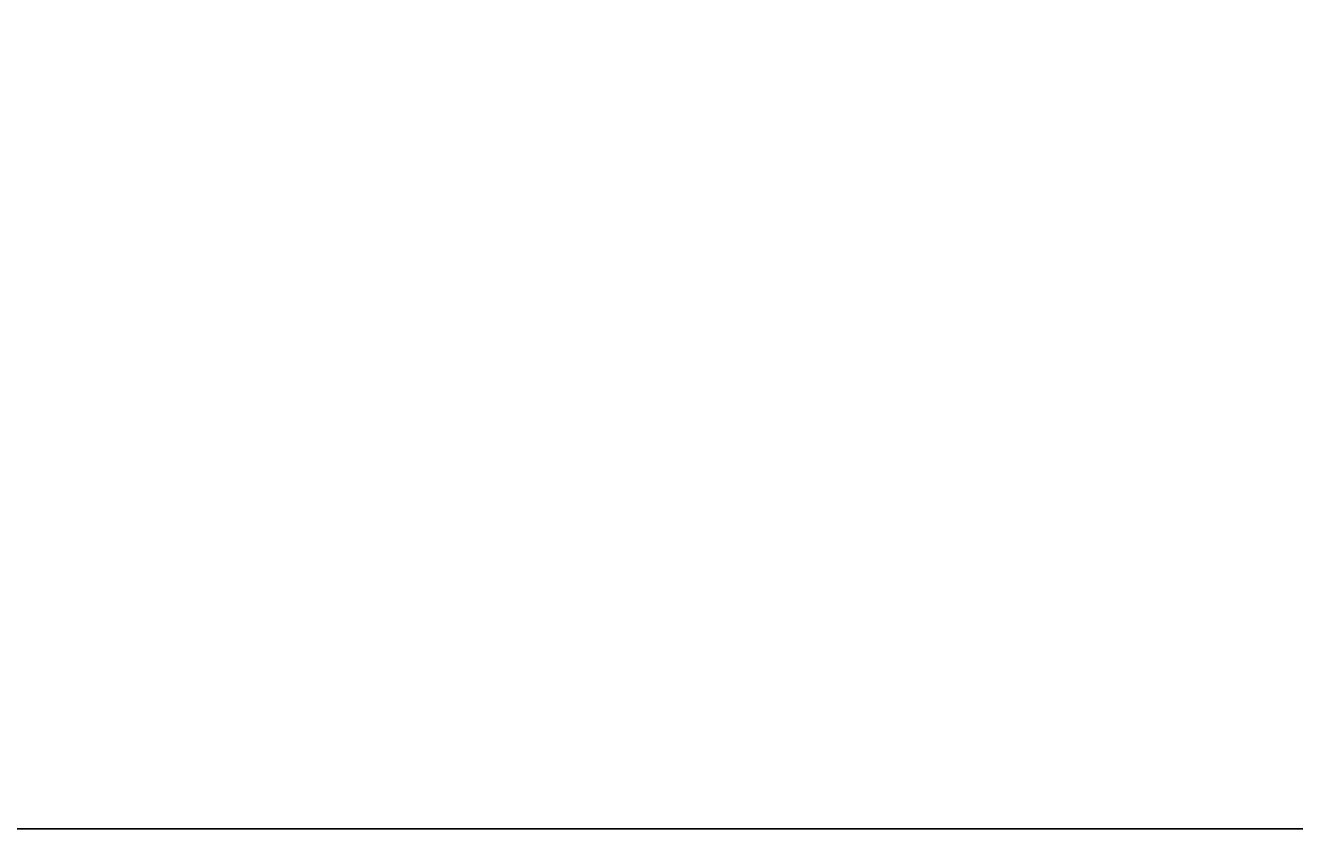
# Model space of a CAD drawing. Units: inches. Extents: x 35362 to 73946, y 43607 to 67532.
# Tile 108 of 134: x 50761 to 50905, y 48969 to 49061. Entities that reach past the tile are written whole.
import ezdxf

# ---------------------------------------------------------------- set-up
doc = ezdxf.new("R2010")
doc.units = ezdxf.units.IN
doc.header["$MEASUREMENT"] = 0
doc.layers.add('A-ANNO-DIMS', color=2, linetype='Continuous', lineweight=18)
doc.styles.get("Standard").update_dxf_attribs({"font": 'arial.ttf'})
doc.dimstyles.get("Standard").update_dxf_attribs({"dimtxt": 0.18, "dimasz": 0.18, "dimexe": 0.18, "dimexo": 0.0625, "dimgap": 0.09, "dimtad": 0, "dimtih": 1, "dimtoh": 1, "dimdec": 4, "dimzin": 0, "dimdsep": 46, "dimtxsty": 'Standard', "dimcen": 0.09, "dimadec": 0, "dimazin": 0, "dimtfac": 1, "dimtdec": 4, "dimtofl": 0, "dimtmove": 0, "dimatfit": 3, "dimfxl": 1, "dimtolj": 1, "dimtzin": 0, "dimarcsym": 0})

# ---------------------------------------------------------------- blocks, each defined once
blk = doc.blocks.new('*D11')
at = {"layer": 'A-ANNO-DIMS', "color": 0, "lineweight": -2, "transparency": 16777216}
for p, q in [((47978.66, 56028.77), (47978.66, 43606.68)), ((53109.76, 56028.77), (53109.76, 43606.68)), ((47978.84, 43606.86), (50543.87, 43606.86)), ((53109.58, 43606.86), (50544.55, 43606.86))]:
    blk.add_line(p, q, dxfattribs=at)
at = {"layer": 'A-ANNO-DIMS', "color": 0, "transparency": 16777216}
for points in [[(47978.84, 43606.89), (47978.84, 43606.83), (47978.66, 43606.86)], [(53109.58, 43606.89), (53109.58, 43606.83), (53109.76, 43606.86)]]:
    blk.add_solid(points, dxfattribs=at)
at = {"layer": 'Defpoints', "color": 0, "transparency": 16777216}
for p in [(47978.66, 56028.84), (53109.76, 56028.84), (53109.76, 43606.86)]:
    blk.add_point(p, dxfattribs=at)
at = {"layer": 'A-ANNO-DIMS', "color": 0, "transparency": 16777216, "insert": (50544.21, 43606.86), "char_height": 0.18, "attachment_point": 5}
blk.add_mtext('\\A1;5131', dxfattribs=at)
blk = doc.blocks.new('*D13')
at = {"layer": 'A-ANNO-DIMS', "color": 0, "lineweight": -2, "transparency": 16777216}
for p, q in [((48373.49, 51694.02), (48373.49, 43606.68)), ((51029.04, 51694.02), (51029.04, 43606.68)), ((48373.67, 43606.86), (49700.8, 43606.86)), ((51028.86, 43606.86), (49701.73, 43606.86))]:
    blk.add_line(p, q, dxfattribs=at)
at = {"layer": 'A-ANNO-DIMS', "color": 0, "transparency": 16777216}
for points in [[(48373.67, 43606.89), (48373.67, 43606.83), (48373.49, 43606.86)], [(51028.86, 43606.89), (51028.86, 43606.83), (51029.04, 43606.86)]]:
    blk.add_solid(points, dxfattribs=at)
at = {"layer": 'Defpoints', "color": 0, "transparency": 16777216}
for p in [(48373.49, 51694.09), (51029.04, 51694.09), (51029.04, 43606.86)]:
    blk.add_point(p, dxfattribs=at)
at = {"layer": 'A-ANNO-DIMS', "color": 0, "transparency": 16777216, "insert": (49701.27, 43606.86), "char_height": 0.18, "attachment_point": 5}
blk.add_mtext('\\A1;2655.6', dxfattribs=at)
blk = doc.blocks.new('*D17')
at = {"layer": 'A-ANNO-DIMS', "color": 0, "lineweight": -2, "transparency": 16777216}
for p, q in [((49923.31, 61293.22), (49923.31, 43606.68)), ((51913.93, 61293.22), (51913.93, 43606.68)), ((49923.49, 43606.86), (50918.16, 43606.86)), ((51913.75, 43606.86), (50919.07, 43606.86))]:
    blk.add_line(p, q, dxfattribs=at)
at = {"layer": 'A-ANNO-DIMS', "color": 0, "transparency": 16777216}
for points in [[(49923.49, 43606.89), (49923.49, 43606.83), (49923.31, 43606.86)], [(51913.75, 43606.89), (51913.75, 43606.83), (51913.93, 43606.86)]]:
    blk.add_solid(points, dxfattribs=at)
at = {"layer": 'Defpoints', "color": 0, "transparency": 16777216}
for p in [(49923.31, 61293.29), (51913.93, 61293.29), (51913.93, 43606.86)]:
    blk.add_point(p, dxfattribs=at)
at = {"layer": 'A-ANNO-DIMS', "color": 0, "transparency": 16777216, "insert": (50918.62, 43606.86), "char_height": 0.18, "attachment_point": 5}
blk.add_mtext('\\A1;1990.6', dxfattribs=at)
blk = doc.blocks.new('*D67')
at = {"layer": 'A-ANNO-DIMS', "color": 0, "lineweight": -2, "transparency": 16777216}
for p, q in [((56873.54, 53351.53), (35361.77, 53351.53)), ((35361.95, 53351.35), (35361.95, 49400.89)), ((35361.95, 45450.07), (35361.95, 49400.53)), ((53793.58, 45449.89), (35361.77, 45449.89))]:
    blk.add_line(p, q, dxfattribs=at)
at = {"layer": 'A-ANNO-DIMS', "color": 0, "transparency": 16777216}
for points in [[(35361.92, 53351.35), (35361.98, 53351.35), (35361.95, 53351.53)], [(35361.92, 45450.07), (35361.98, 45450.07), (35361.95, 45449.89)]]:
    blk.add_solid(points, dxfattribs=at)
at = {"layer": 'Defpoints', "color": 0, "transparency": 16777216}
for p in [(35361.95, 53351.53), (56873.6, 53351.53), (53793.64, 45449.89)]:
    blk.add_point(p, dxfattribs=at)
at = {"layer": 'A-ANNO-DIMS', "color": 0, "transparency": 16777216, "insert": (35361.95, 49400.71), "char_height": 0.18, "attachment_point": 5}
blk.add_mtext('\\A1;7901.6', dxfattribs=at)
blk = doc.blocks.new('*D84')
at = {"layer": 'A-ANNO-DIMS', "color": 0, "lineweight": -2, "transparency": 16777216}
for p, q in [((55540.23, 49259.94), (35361.77, 49259.94)), ((35361.95, 49259.76), (35361.95, 49115.14)), ((35361.95, 48970.16), (35361.95, 49114.78)), ((55540.23, 48969.98), (35361.77, 48969.98))]:
    blk.add_line(p, q, dxfattribs=at)
at = {"layer": 'A-ANNO-DIMS', "color": 0, "transparency": 16777216}
for points in [[(35361.92, 49259.76), (35361.98, 49259.76), (35361.95, 49259.94)], [(35361.92, 48970.16), (35361.98, 48970.16), (35361.95, 48969.98)]]:
    blk.add_solid(points, dxfattribs=at)
at = {"layer": 'Defpoints', "color": 0, "transparency": 16777216}
for p in [(35361.95, 49259.94), (55540.3, 49259.94), (55540.3, 48969.98)]:
    blk.add_point(p, dxfattribs=at)
at = {"layer": 'A-ANNO-DIMS', "color": 0, "transparency": 16777216, "insert": (35361.95, 49114.96), "char_height": 0.18, "attachment_point": 5}
blk.add_mtext('\\A1;289.96', dxfattribs=at)
blk = doc.blocks.new('*D86')
at = {"layer": 'A-ANNO-DIMS', "color": 0, "lineweight": -2, "transparency": 16777216}
for p, q in [((51285.53, 49320.08), (35361.77, 49320.08)), ((35361.95, 49319.9), (35361.95, 49120.26)), ((35361.95, 48920.26), (35361.95, 49119.9)), ((51285.53, 48920.08), (35361.77, 48920.08))]:
    blk.add_line(p, q, dxfattribs=at)
at = {"layer": 'A-ANNO-DIMS', "color": 0, "transparency": 16777216}
for points in [[(35361.92, 49319.9), (35361.98, 49319.9), (35361.95, 49320.08)], [(35361.92, 48920.26), (35361.98, 48920.26), (35361.95, 48920.08)]]:
    blk.add_solid(points, dxfattribs=at)
at = {"layer": 'Defpoints', "color": 0, "transparency": 16777216}
for p in [(35361.95, 49320.08), (51285.59, 49320.08), (51285.59, 48920.08)]:
    blk.add_point(p, dxfattribs=at)
at = {"layer": 'A-ANNO-DIMS', "color": 0, "transparency": 16777216, "insert": (35361.95, 49120.08), "char_height": 0.18, "attachment_point": 5}
blk.add_mtext('\\A1;400.0', dxfattribs=at)
blk = doc.blocks.new('*D107')
at = {"layer": 'A-ANNO-DIMS', "color": 0, "lineweight": -2, "transparency": 16777216}
for p, q in [((50139.56, 59850.01), (50139.56, 43606.68)), ((51320.81, 59850.01), (51320.81, 43606.68)), ((50139.74, 43606.86), (50729.73, 43606.86)), ((51320.63, 43606.86), (50730.64, 43606.86))]:
    blk.add_line(p, q, dxfattribs=at)
at = {"layer": 'A-ANNO-DIMS', "color": 0, "transparency": 16777216}
for points in [[(50139.74, 43606.89), (50139.74, 43606.83), (50139.56, 43606.86)], [(51320.63, 43606.89), (51320.63, 43606.83), (51320.81, 43606.86)]]:
    blk.add_solid(points, dxfattribs=at)
at = {"layer": 'Defpoints', "color": 0, "transparency": 16777216}
for p in [(50139.56, 59850.08), (51320.81, 59850.08), (51320.81, 43606.86)]:
    blk.add_point(p, dxfattribs=at)
at = {"layer": 'A-ANNO-DIMS', "color": 0, "transparency": 16777216, "insert": (50730.19, 43606.86), "char_height": 0.18, "attachment_point": 5}
blk.add_mtext('\\A1;1181.3', dxfattribs=at)

msp = doc.modelspace()

# ---------------------------------------------------------------- dimensions: what is measured, and where the dimension line sits
at = {"layer": 'A-ANNO-DIMS'}
for base, p1, p2, override, picture, middle in [((51913.931, 43606.859), (49923.307, 61293.286), (51913.931, 61293.286), {"dimdec": 1, "dimlfac": 1, "dimrnd": 0, "dimzin": 0, "dimdsep": 46, "dimlunit": 2}, '*D17', (50918.619, 43606.859)), ((51320.8133, 43606.859), (50139.5627, 59850.0769), (51320.8133, 59850.0769), {"dimdec": 1, "dimlfac": 1, "dimrnd": 0, "dimzin": 0, "dimdsep": 46, "dimlunit": 2}, '*D107', (50730.188, 43606.859)), ((53109.76, 43606.859), (47978.665, 56028.836), (53109.76, 56028.836), {"dimdec": 0, "dimlfac": 1, "dimrnd": 0, "dimzin": 0, "dimdsep": 46, "dimlunit": 2}, '*D11', (50544.212, 43606.859)), ((51029.043, 43606.859), (48373.492, 51694.087), (51029.043, 51694.087), {"dimdec": 1, "dimlfac": 1, "dimrnd": 0, "dimzin": 0, "dimdsep": 46, "dimlunit": 2}, '*D13', (49701.267, 43606.859))]:
    dim = msp.add_linear_dim(base=base, p1=p1, p2=p2, dimstyle='Standard', override=override, dxfattribs=at)
    dim.commit()
    dim.dimension.update_dxf_attribs({"geometry": picture, "text_midpoint": middle})
for base, p1, p2, override, picture, middle in [((35361.949, 53351.529), (53793.638, 45449.894), (56873.602, 53351.529), {"dimdec": 1, "dimlfac": 1, "dimrnd": 0, "dimzin": 0, "dimdsep": 46, "dimlunit": 2}, '*D67', (35361.949, 49400.712)), ((35361.949, 49320.079), (51285.595, 48920.079), (51285.595, 49320.079), {"dimdec": 1, "dimlfac": 1, "dimrnd": 0, "dimzin": 0, "dimdsep": 46, "dimlunit": 2}, '*D86', (35361.949, 49120.079)), ((35361.9491, 49259.9353), (55540.2972, 48969.9796), (55540.2972, 49259.9353), {"dimdec": 2, "dimlfac": 1, "dimrnd": 0, "dimzin": 0, "dimdsep": 46, "dimlunit": 2}, '*D84', (35361.9491, 49114.9575))]:
    dim = msp.add_linear_dim(base=base, p1=p1, p2=p2, angle=90, dimstyle='Standard', override=override, dxfattribs=at)
    dim.commit()
    dim.dimension.update_dxf_attribs({"geometry": picture, "text_midpoint": middle})

doc.saveas('drawing.dxf')
